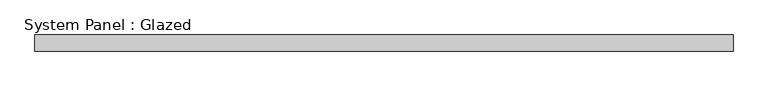
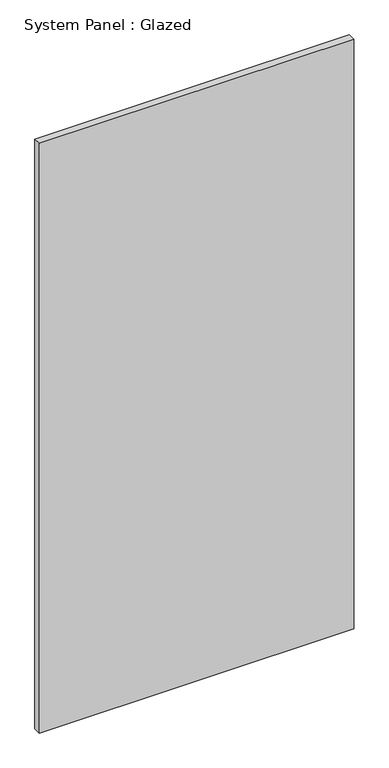
"""IFC4 building model written with IfcOpenShell, lengths in millimetres: plate geometry, System Panel : Glazed."""

from ifc_helpers import new_model, si_unit, origin, origin_with_axes, place, context, project, spatial, polyline, outline, extrude, source, transform, mapped, element, save


def system_panel_glazed_a9a9195b(model_context):
    return source(origin(), model_context, "Body", "SweptSolid", [
        extrude(outline(polyline([(536.575, 19.05), (-536.575, 19.05), (-536.575, 44.45), (536.575, 44.45), (536.575, 19.05)])), origin_with_axes(), (0.0, 0.0, 1.0), 2127.3645985),
    ])


if __name__ == "__main__":
    model = new_model("IFC4")
    model_context = context("Model", 3, world=origin())
    ifc_project = project(units=[si_unit("LENGTHUNIT", "METRE", prefix="MILLI")], contexts=[model_context])
    site = spatial("IfcSite", under=ifc_project)
    building = spatial("IfcBuilding", under=site)
    placement = place(None, origin())
    system_panel_glazed_shape = system_panel_glazed_a9a9195b(model_context)
    element("IfcPlate", 1, ObjectType="System Panel : Glazed", at=placement, inside=building, context=model_context, shape_type="MappedRepresentation", body=[
        mapped(system_panel_glazed_shape, transform((0.0, 0.0, 0.0), x_axis=(1.0, 0.0, 0.0), y_axis=(0.0, 1.0, 0.0), z_axis=(0.0, 0.0, 1.0))),
    ])
    save(model, "model.ifc")

# Revit data of these elements
# Type "System Panel : Glazed"
#   Construction Type Id = "GSP4R"
#   Analytic Construction = "1/8 in Pilkington single glazing"
#   Visual Light Transmittance = 0.9
#   Solar Heat Gain Coefficient = 0.86
#   Heat Transfer Coefficient (U) = 1.18115 BTU/(h·ft²·°F)
#   Define Thermal Properties by = 1
# Element 1 (IfcPlate, "System Panel : Glazed")
#   Materials on its faces: "Glass"
# Materials
#   "Glass": class "Glass", colour RGB 0 128 192, transparency 0.75, Description = "Soda Lime Glass", Cost = 0
